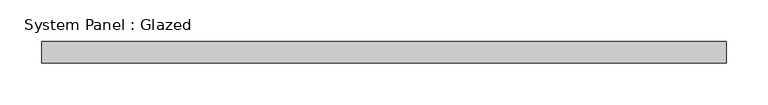
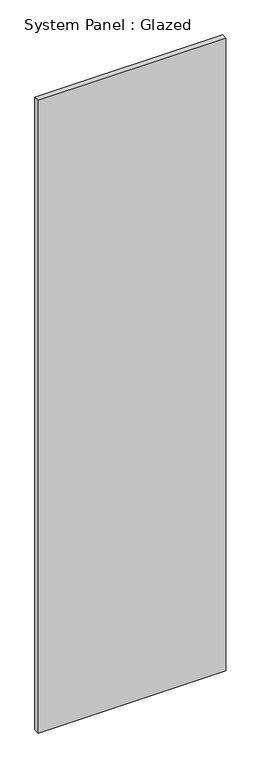
"""IFC4 building model written with IfcOpenShell, lengths in millimetres: plate geometry, System Panel : Glazed."""

from ifc_helpers import new_model, si_unit, origin, origin_with_axes, place, context, project, spatial, polyline, outline, extrude, source, transform, mapped, element, save


def system_panel_glazed_52d31088(model_context):
    return source(origin(), model_context, "Body", "SweptSolid", [
        extrude(outline(polyline([(409.575, 19.05), (-409.575, 19.05), (-409.575, 44.45), (409.575, 44.45), (409.575, 19.05)])), origin_with_axes(), (0.0, 0.0, 1.0), 2921.0),
    ])


if __name__ == "__main__":
    model = new_model("IFC4")
    model_context = context("Model", 3, world=origin())
    ifc_project = project(units=[si_unit("LENGTHUNIT", "METRE", prefix="MILLI")], contexts=[model_context])
    site = spatial("IfcSite", under=ifc_project)
    building = spatial("IfcBuilding", under=site)
    placement = place(None, origin())
    system_panel_glazed_shape = system_panel_glazed_52d31088(model_context)
    element("IfcPlate", 1, ObjectType="System Panel : Glazed", at=placement, inside=building, context=model_context, shape_type="MappedRepresentation", body=[
        mapped(system_panel_glazed_shape, transform((0.0, 0.0, 0.0), x_axis=(1.0, 0.0, 0.0), y_axis=(0.0, 1.0, 0.0), z_axis=(0.0, 0.0, 1.0))),
    ])
    save(model, "model.ifc")

# Revit data of these elements
# Type "System Panel : Glazed"
#   Construction Type Id = "GSP4R"
#   Analytic Construction = "1/8 in Pilkington single glazing"
#   Visual Light Transmittance = 0.9
#   Solar Heat Gain Coefficient = 0.86
#   Heat Transfer Coefficient (U) = 1.18115 BTU/(h·ft²·°F)
# Element 1 (IfcPlate, "System Panel : Glazed")
#   Materials on its faces: "Glass"
# Materials
#   "Glass": class "Glass", colour RGB 0 128 192, transparency 0.75, Description = "Soda Lime Glass", Cost = 0
